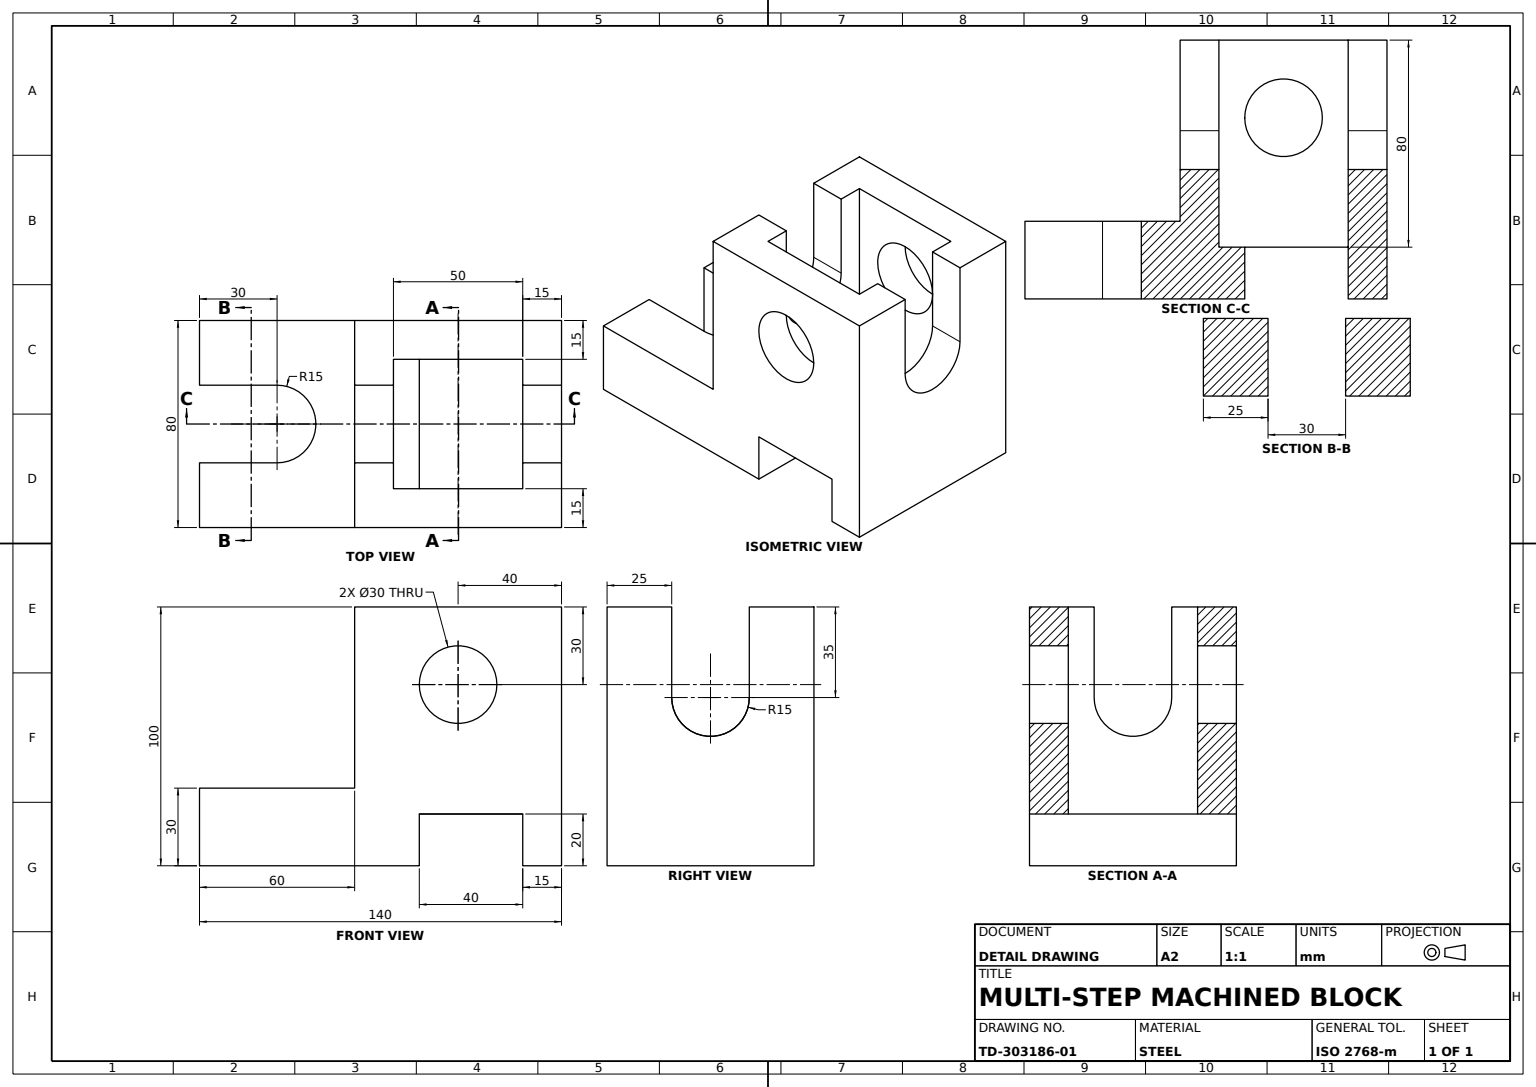
SolidWorks part; units mm, degrees
material "Plain Carbon Steel"
ref_plane "Front Plane" through (0, 0, 0) normal (0, 0, 1) x (1, 0, 0)
ref_plane "Top Plane" through (0, 0, 0) normal (0, 1, 0) x (1, 0, 0)
ref_plane "Right Plane" through (0, 0, 0) normal (1, 0, 0) x (0, 0, -1)
sketch "Base Block Sketch" plane through (0, 0, 0) normal (0, 0, 1) x (1, 0, 0)
  line L0 (0, 0) -> (0, 30)
  line L1 (0, 30) -> (140, 30)
  line L2 (140, 30) -> (140, 0)
  line L3 (140, 0) -> (0, 0)
  dimension "D1" = 30
  dimension "D2" = 140
  dimension "D3" = 30
extrude "Base Block" add sketch "Base Block Sketch" against normal blind 80
sketch "Base Notch Sketch" plane through (0, 0, 0) normal (0, 0, 1) x (1, 0, 0)
  line L0 (140, 0) -> (140, 20)
  line L1 (140, 0) -> (140, 30) construction
  line L3 (125, 20) -> (85, 20)
  line L4 (85, 20) -> (85, 0)
  line L5 (0, 0) -> (140, 0) construction
  line L6 (85, 0) -> (125, 0)
  line L7 (125, 0) -> (125, 20)
  line M3 (0, 0) -> (140, 0)
  dimension "D1" = 20
  dimension "D2" = 15
  dimension "D3" = 40
  dimension "D4" = 40
  dimension "D5" = 20
extrude "Base Notch" cut sketch "Base Notch Sketch" against normal blind 80 contours L7 L3 L4 M3
sketch "Upright Sketch" plane through (0, 0, 0) normal (0, 0, 1) x (1, 0, 0)
  line L0 (140, 30) -> (140, 100)
  line L1 (140, 100) -> (60, 100)
  line L2 (60, 100) -> (60, 30)
  line L3 (140, 30) -> (0, 30) construction
  line L4 (60, 30) -> (140, 30)
  dimension "D1" = 70
  dimension "D2" = 80
extrude "Upright" add sketch "Upright Sketch" against normal blind 80
sketch "Upright Profile Cut Sketch" plane through (0, 100, 0) normal (0, 1, 0) x (1, 0, 0)
  line L0 (60, 40) -> (75, 40)
  line L1 (60, 80) -> (60, 0) construction
  line L2 (75, 40) -> (75, 65)
  line L3 (75, 65) -> (125, 65)
  line L4 (125, 65) -> (125, 15)
  line L5 (125, 15) -> (75, 15)
  line L6 (75, 15) -> (75, 40)
  dimension "D1" = 15
  dimension "D2" = 25
  dimension "D3" = 50
  dimension "D4" = 50
  dimension "D5" = 50
extrude "Upright Profile Cut" cut sketch "Upright Profile Cut Sketch" against normal blind 80 contours L6 L5 L4 L3 L2
sketch "Cross Hole Sketch" plane through (0, 0, 0) normal (0, 0, 1) x (1, 0, 0)
  line L0 (100, 100) -> (100, 70)
  line L1 (140, 100) -> (60, 100) construction
  circle A0 centre (100, 70) radius 15
  dimension "D2" = 30
  dimension "D1" = 30
extrude "Cross Hole" cut sketch "Cross Hole Sketch" against normal blind 80
sketch "Upright U-Slot Sketch" plane through (60, 0, 0) normal (-1, 0, 0) x (0, 0, 1)
  line L0 (-40, 100) -> (-40, 65)
  line L1 (-80, 100) -> (0, 100) construction
  line L2 (-55, 65) -> (-55, 100)
  line L3 (-55, 100) -> (-25, 100)
  line L4 (-25, 100) -> (-25, 65)
  circle A0 centre (-40, 65) radius 15
  dimension "D2" = 15
  dimension "D1" = 35
extrude "Upright U-Slot" cut sketch "Upright U-Slot Sketch" against normal blind 80
sketch "Base Underside Notch Sketch" plane through (0, 30, 0) normal (0, 1, 0) x (1, 0, 0)
  line L0 (0, 40) -> (30, 40)
  line L1 (0, 80) -> (0, 0) construction
  line L2 (30, 55) -> (0, 55)
  line L3 (0, 55) -> (0, 25)
  line L4 (0, 25) -> (30, 25)
  arc A0 (30, 25) -> (30, 55) centre (30, 40) ccw
  dimension "D2" = 15
  dimension "D1" = 30
  dimension "D3" = 30
  dimension "D4" = 30
  dimension "D5" = 30
  dimension "D6" = 30
extrude "Base Underside Notch" cut sketch "Base Underside Notch Sketch" against normal blind 80 and the other way blind 10
